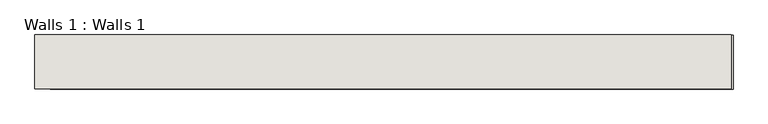
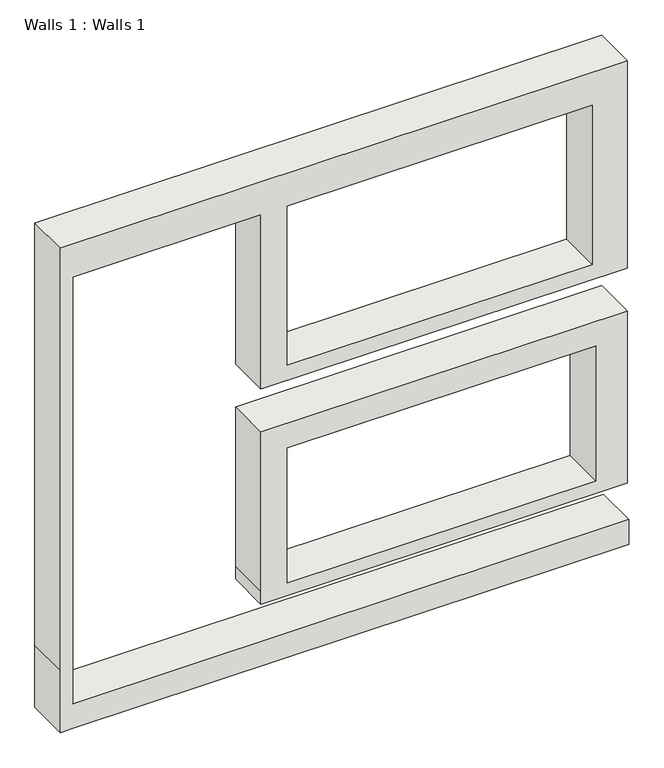
"""IFC4 building model written with IfcOpenShell, lengths in millimetres: wall geometry, Walls 1 : Walls 1."""

from ifc_helpers import new_model, si_unit, frame, origin, place, context, project, spatial, polyline, outline, extrude, source, transform, mapped, element, save


def walls_1_walls_1_cc25df17(model_context):
    return source(origin(), model_context, "Body", "SweptSolid", [
        extrude(outline(polyline([(3835.4, -7651.4936733), (10744.2, -7651.4936733), (10744.2, -4388.0195107), (7543.8, -4388.0195107), (7543.8, 1962.4063267), (10744.2, 1962.4063267), (11349.3315531, 1962.4063267), (11349.3315531, -7867.8195107), (3606.8, -7867.8195107), (2463.8, -7867.8195107), (2463.8, -7651.4936733), (2463.8, 1986.1481409), (2921.0, 1986.1481409), (2921.0, -7651.4936733), (3835.4, -7651.4936733)]), holes=[polyline([(7823.2, 1352.3804893), (7823.2, -3930.3936733), (10744.2, -3930.3936733), (10744.2, 1352.3804893), (7823.2, 1352.3804893)])]), frame((0.0, 3150.9419215, 0.0), z_axis=(0.0, 1.0, 0.0), x_axis=(0.0, 0.0, 1.0)), (0.0, 0.0, 1.0), 762.0),
        extrude(outline(polyline([(6756.4, 1962.4063267), (6756.4, -4388.0195107), (3835.4, -4388.0195107), (3600.45, -4388.0195107), (3600.45, 1962.4063267), (6756.4, 1962.4063267)]), holes=[polyline([(6308.7777042, 1411.8513632), (3835.4, 1411.8513632), (3835.4, -3930.3936733), (6308.7777042, -3930.3936733), (6308.7777042, 1411.8513632)])]), frame((0.0, 3150.9419215, 0.0), z_axis=(0.0, 1.0, 0.0), x_axis=(0.0, 0.0, 1.0)), (0.0, 0.0, 1.0), 762.0),
    ])


if __name__ == "__main__":
    model = new_model("IFC4")
    model_context = context("Model", 3, world=origin())
    ifc_project = project(units=[si_unit("LENGTHUNIT", "METRE", prefix="MILLI")], contexts=[model_context])
    site = spatial("IfcSite", under=ifc_project)
    building = spatial("IfcBuilding", under=site)
    placement = place(None, origin())
    walls_1_walls_1_shape = walls_1_walls_1_cc25df17(model_context)
    element("IfcWall", 1, ObjectType="Walls 1 : Walls 1", at=placement, inside=building, context=model_context, shape_type="MappedRepresentation", body=[
        mapped(walls_1_walls_1_shape, transform((0.0, 0.0, 0.0), x_axis=(1.0, 0.0, 0.0), y_axis=(0.0, 1.0, 0.0), z_axis=(0.0, 0.0, 1.0))),
    ])
    save(model, "model.ifc")

# Revit data of these elements
# Element 1 (IfcWall, "Walls 1 : Walls 1")
#   Materials on its faces: "Default Wall"
# Materials
#   "Default Wall": colour RGB 128 128 128, transparency 0
